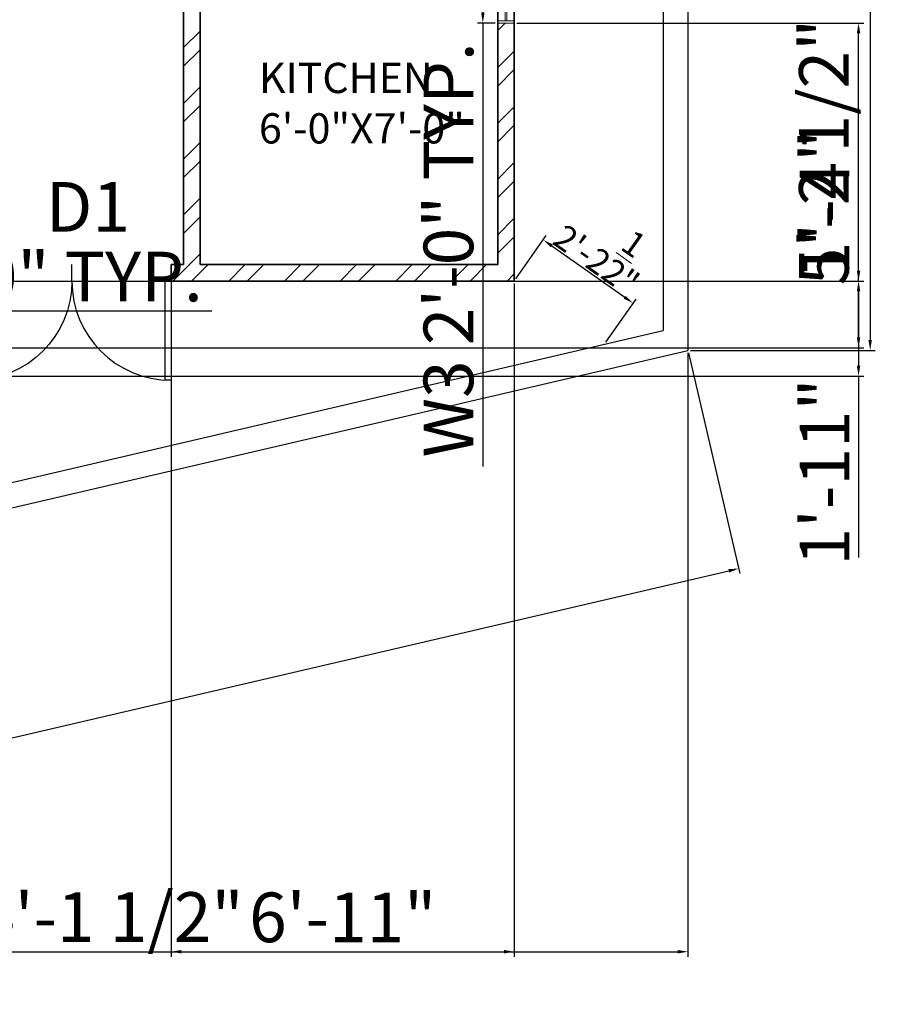
# Model space of a CAD drawing. Units: inches. Extents: x 2242 to 2870, y 1782 to 2635.
# Tile 3 of 7: x 2594 to 2807, y 1782 to 2020. Entities that reach past the tile are written whole.
import ezdxf

# ---------------------------------------------------------------- set-up
doc = ezdxf.new("R2010")
doc.units = ezdxf.units.IN
for name, color, linetype, lineweight in [('A-ANNO-DIMS', 7, 'Continuous', 18), ('A-ANNO-TEXT', 1, 'Continuous', 18), ('A-AREA-IDEN', 1, 'Continuous', 25), ('A-WALL-PATT', 253, 'Continuous', 13), ('C-PROP', 7, 'Continuous', 30), ('doors', 5, 'Continuous', 25), ('walls', 7, 'Continuous', 35), ('windows', 72, 'Continuous', 18)]:
    doc.layers.add(name, color=color, linetype=linetype, lineweight=lineweight)
doc.styles.get("Standard").update_dxf_attribs({"font": 'arial.ttf'})
doc.dimstyles.new('ISO-25', dxfattribs={"dimtxt": 12, "dimasz": 2.5, "dimexe": 1.25, "dimexo": 0.625, "dimtad": 1, "dimlunit": 4, "dimtxsty": 'Standard', "dimcen": 2.5, "dimadec": 0, "dimazin": 0, "dimtfac": 1, "dimtmove": 0, "dimatfit": 3, "dimfxl": 1, "dimarcsym": 0})

# ---------------------------------------------------------------- blocks, each defined once
blk = doc.blocks.new('*U2')
for p, q in [((0, 0), (0, -5)), ((30, 0), (30, -5))]:
    blk.add_line(p, q)
blk.add_lwpolyline([(0, 0), (0, 30), (1.75, 30), (1.75, 0)], close=True)
blk.add_arc((0, 0), 30, 0, 90)
blk = doc.blocks.new('*D17')
at = {"layer": 'A-ANNO-DIMS', "color": 0, "lineweight": -2, "transparency": 16777216}
for p, q in [((2755.31, 1939.73), (2767.74, 1886.37)), ((2322.86, 1784), (2765.02, 1887.02)), ((2308.28, 1835.57), (2320.71, 1782.21))]:
    blk.add_line(p, q, dxfattribs=at)
at = {"layer": 'A-ANNO-DIMS', "color": 0, "transparency": 16777216}
for points in [[(2764.92, 1887.42), (2765.11, 1886.61), (2767.45, 1887.58)], [(2322.77, 1784.4), (2322.96, 1783.59), (2320.43, 1783.43)]]:
    blk.add_solid(points, dxfattribs=at)
at = {"layer": 'Defpoints', "color": 0, "transparency": 16777216}
for p in [(2755.16, 1940.33), (2767.45, 1887.58), (2308.14, 1836.18)]:
    blk.add_point(p, dxfattribs=at)
at = {"layer": 'A-ANNO-DIMS', "color": 0, "transparency": 16777216, "insert": (2542.41, 1842.09), "char_height": 12, "attachment_point": 5, "rotation": 13.1155}
blk.add_mtext('38\'-3"', dxfattribs=at)
blk = doc.blocks.new('*D19')
at = {"layer": 'A-ANNO-DIMS', "color": 0, "lineweight": -2, "transparency": 16777216}
for p, q in [((2713.52, 1957.61), (2720.9, 1968.07)), ((2722.22, 1965.61), (2739.87, 1953.17)), ((2735.26, 1942.28), (2742.64, 1952.75))]:
    blk.add_line(p, q, dxfattribs=at)
at = {"layer": 'A-ANNO-DIMS', "color": 0, "transparency": 16777216}
for points in [[(2722.46, 1965.95), (2721.98, 1965.27), (2720.18, 1967.05)], [(2740.11, 1953.51), (2739.63, 1952.83), (2741.92, 1951.73)]]:
    blk.add_solid(points, dxfattribs=at)
at = {"layer": 'Defpoints', "color": 0, "transparency": 16777216}
for p in [(2713.16, 1957.1), (2741.92, 1951.73), (2734.9, 1941.77)]:
    blk.add_point(p, dxfattribs=at)
at = {"layer": 'A-ANNO-DIMS', "color": 0, "transparency": 16777216, "insert": (2735.46, 1965.64), "char_height": 6, "attachment_point": 5, "rotation": 324.8144}
blk.add_mtext('2\'-2{\\H1x;\\S1/2;}"', dxfattribs=at)
blk = doc.blocks.new('*D29')
at = {"layer": 'A-ANNO-DIMS', "color": 0, "lineweight": -2, "transparency": 16777216}
for p, q in [((2755.79, 2540.33), (2800.47, 2540.33)), ((2799.22, 2537.83), (2799.22, 1942.83)), ((2755.79, 1940.33), (2800.47, 1940.33))]:
    blk.add_line(p, q, dxfattribs=at)
at = {"layer": 'A-ANNO-DIMS', "color": 0, "transparency": 16777216}
for points in [[(2798.81, 2537.83), (2799.64, 2537.83), (2799.22, 2540.33)], [(2798.81, 1942.83), (2799.64, 1942.83), (2799.22, 1940.33)]]:
    blk.add_solid(points, dxfattribs=at)
at = {"layer": 'Defpoints', "color": 0, "transparency": 16777216}
for p in [(2755.16, 2540.33), (2755.16, 1940.33), (2799.22, 1940.33)]:
    blk.add_point(p, dxfattribs=at)
at = {"layer": 'A-ANNO-DIMS', "color": 0, "transparency": 16777216, "insert": (2792.47, 2240.33), "char_height": 12, "attachment_point": 5, "rotation": 90}
blk.add_mtext("50'", dxfattribs=at)
blk = doc.blocks.new('WIN-W3-24IN')
for p, q in [((0, 0), (0, 24.12)), ((0, 24.12), (4, 24.12)), ((4, 24.12), (4, 0)), ((0, 23.62), (4, 23.62)), ((1.8, 23.62), (1.8, 0.5)), ((2.2, 23.62), (2.2, 0.5)), ((4, 0.5), (0, 0.5)), ((4, 0), (0, 0))]:
    blk.add_line(p, q)
blk = doc.blocks.new('*D35')
at = {"layer": 'A-ANNO-DIMS', "color": 0, "lineweight": -2, "transparency": 16777216}
for p, q in [((2484.67, 1956.47), (2484.67, 1948.63)), ((2532.79, 1956.47), (2532.79, 1948.63)), ((2487.17, 1949.88), (2530.29, 1949.88)), ((2532.79, 1949.88), (2639.98, 1949.88))]:
    blk.add_line(p, q, dxfattribs=at)
at = {"layer": 'A-ANNO-DIMS', "color": 0, "transparency": 16777216}
for points in [[(2487.17, 1950.3), (2487.17, 1949.46), (2484.67, 1949.88)], [(2530.29, 1950.3), (2530.29, 1949.46), (2532.79, 1949.88)]]:
    blk.add_solid(points, dxfattribs=at)
at = {"layer": 'Defpoints', "color": 0, "transparency": 16777216}
for p in [(2484.67, 1957.1), (2532.79, 1957.1), (2532.79, 1949.88)]:
    blk.add_point(p, dxfattribs=at)
at = {"layer": 'A-ANNO-DIMS', "color": 0, "transparency": 16777216, "insert": (2587.64, 1956.63), "char_height": 12, "attachment_point": 5}
blk.add_mtext('W1 4\'-0" TYP.', dxfattribs=at)
blk = doc.blocks.new('*D37')
at = {"layer": 'A-ANNO-DIMS', "color": 0, "lineweight": -2, "transparency": 16777216}
for p, q in [((2708.54, 2043.59), (2704.3, 2043.59)), ((2705.55, 2041.09), (2705.55, 2021.98)), ((2708.54, 2019.48), (2704.3, 2019.48)), ((2705.55, 2019.48), (2705.55, 1912.29))]:
    blk.add_line(p, q, dxfattribs=at)
at = {"layer": 'A-ANNO-DIMS', "color": 0, "transparency": 16777216}
for points in [[(2705.13, 2041.09), (2705.96, 2041.09), (2705.55, 2043.59)], [(2705.13, 2021.98), (2705.96, 2021.98), (2705.55, 2019.48)]]:
    blk.add_solid(points, dxfattribs=at)
at = {"layer": 'Defpoints', "color": 0, "transparency": 16777216}
for p in [(2709.16, 2043.59), (2705.55, 2019.48), (2709.16, 2019.48)]:
    blk.add_point(p, dxfattribs=at)
at = {"layer": 'A-ANNO-DIMS', "color": 0, "transparency": 16777216, "insert": (2698.79, 1964.63), "char_height": 12, "attachment_point": 5, "rotation": 90}
blk.add_mtext('W3 2\'-0" TYP.', dxfattribs=at)
blk = doc.blocks.new('*D42')
at = {"layer": 'A-ANNO-DIMS', "color": 0, "lineweight": -2, "transparency": 16777216}
for p, q in [((2522.93, 2020.21), (2522.93, 2026.94)), ((2537.42, 2020.21), (2537.42, 2026.94)), ((2525.43, 2025.69), (2534.92, 2025.69)), ((2537.42, 2025.69), (2641.15, 2025.69))]:
    blk.add_line(p, q, dxfattribs=at)
at = {"layer": 'A-ANNO-DIMS', "color": 0, "transparency": 16777216}
for points in [[(2525.43, 2026.11), (2525.43, 2025.28), (2522.93, 2025.69)], [(2534.92, 2026.11), (2534.92, 2025.28), (2537.42, 2025.69)]]:
    blk.add_solid(points, dxfattribs=at)
at = {"layer": 'Defpoints', "color": 0, "transparency": 16777216}
for p in [(2537.42, 2025.69), (2522.93, 2019.58), (2537.42, 2019.58)]:
    blk.add_point(p, dxfattribs=at)
at = {"layer": 'A-ANNO-DIMS', "color": 0, "transparency": 16777216, "insert": (2590.54, 2032.52), "char_height": 12, "attachment_point": 5}
blk.add_mtext('1\'-2 1/2" TYP.', dxfattribs=at)
blk = doc.blocks.new('*D56')
at = {"layer": 'A-ANNO-DIMS', "color": 0, "lineweight": -2, "transparency": 16777216}
for p, q in [((2755.16, 1939.71), (2755.16, 1793.68)), ((2308.14, 1835.56), (2308.14, 1793.68)), ((2310.64, 1794.93), (2752.66, 1794.93))]:
    blk.add_line(p, q, dxfattribs=at)
at = {"layer": 'A-ANNO-DIMS', "color": 0, "transparency": 16777216}
for points in [[(2310.64, 1795.35), (2310.64, 1794.51), (2308.14, 1794.93)], [(2752.66, 1795.35), (2752.66, 1794.51), (2755.16, 1794.93)]]:
    blk.add_solid(points, dxfattribs=at)
at = {"layer": 'Defpoints', "color": 0, "transparency": 16777216}
for p in [(2755.16, 1940.33), (2308.14, 1836.18), (2755.16, 1794.93)]:
    blk.add_point(p, dxfattribs=at)
at = {"layer": 'A-ANNO-DIMS', "color": 0, "transparency": 16777216, "insert": (2531.65, 1801.69), "char_height": 12, "attachment_point": 5}
blk.add_mtext('37\'-3"', dxfattribs=at)
blk = doc.blocks.new('*D57')
at = {"layer": 'A-ANNO-DIMS', "color": 0, "lineweight": -2, "transparency": 16777216}
for p, q in [((2713.16, 1956.47), (2713.16, 1793.68)), ((2388.74, 1896.47), (2388.74, 1793.68)), ((2391.24, 1794.93), (2710.66, 1794.93))]:
    blk.add_line(p, q, dxfattribs=at)
at = {"layer": 'A-ANNO-DIMS', "color": 0, "transparency": 16777216}
for points in [[(2391.24, 1795.35), (2391.24, 1794.51), (2388.74, 1794.93)], [(2710.66, 1795.35), (2710.66, 1794.51), (2713.16, 1794.93)]]:
    blk.add_solid(points, dxfattribs=at)
at = {"layer": 'Defpoints', "color": 0, "transparency": 16777216}
for p in [(2713.16, 1957.1), (2388.74, 1897.1), (2713.16, 1794.93)]:
    blk.add_point(p, dxfattribs=at)
at = {"layer": 'A-ANNO-DIMS', "color": 0, "transparency": 16777216, "insert": (2550.95, 1801.76), "char_height": 12, "attachment_point": 5}
blk.add_mtext('27\'-0 1/2"', dxfattribs=at)
blk = doc.blocks.new('*D68')
at = {"layer": 'A-ANNO-DIMS', "color": 0, "lineweight": -2, "transparency": 16777216}
for p, q in [((2713.79, 2019.48), (2797.66, 2019.48)), ((2796.41, 1959.6), (2796.41, 2016.98)), ((2713.79, 1957.1), (2797.66, 1957.1))]:
    blk.add_line(p, q, dxfattribs=at)
at = {"layer": 'A-ANNO-DIMS', "color": 0, "transparency": 16777216}
for points in [[(2796, 2016.98), (2796.83, 2016.98), (2796.41, 2019.48)], [(2796, 1959.6), (2796.83, 1959.6), (2796.41, 1957.1)]]:
    blk.add_solid(points, dxfattribs=at)
at = {"layer": 'Defpoints', "color": 0, "transparency": 16777216}
for p in [(2713.16, 2019.48), (2796.41, 2019.48), (2713.16, 1957.1)]:
    blk.add_point(p, dxfattribs=at)
at = {"layer": 'A-ANNO-DIMS', "color": 0, "transparency": 16777216, "insert": (2789.58, 1988.29), "char_height": 12, "attachment_point": 5, "rotation": 90}
blk.add_mtext('5\'-2 1/2"', dxfattribs=at)
blk = doc.blocks.new('*D72')
at = {"layer": 'A-ANNO-DIMS', "color": 0, "lineweight": -2, "transparency": 16777216}
for p, q in [((2532.79, 1956.47), (2532.79, 1793.68)), ((2582.16, 1956.47), (2582.16, 1793.68)), ((2535.29, 1794.93), (2579.66, 1794.93)), ((2582.16, 1794.93), (2646.26, 1794.93))]:
    blk.add_line(p, q, dxfattribs=at)
at = {"layer": 'A-ANNO-DIMS', "color": 0, "transparency": 16777216}
for points in [[(2535.29, 1795.35), (2535.29, 1794.51), (2532.79, 1794.93)], [(2579.66, 1795.35), (2579.66, 1794.51), (2582.16, 1794.93)]]:
    blk.add_solid(points, dxfattribs=at)
at = {"layer": 'Defpoints', "color": 0, "transparency": 16777216}
for p in [(2532.79, 1957.1), (2582.16, 1957.1), (2582.16, 1794.93)]:
    blk.add_point(p, dxfattribs=at)
at = {"layer": 'A-ANNO-DIMS', "color": 0, "transparency": 16777216, "insert": (2615.46, 1801.76), "char_height": 12, "attachment_point": 5}
blk.add_mtext('4\'-1 1/2"', dxfattribs=at)
blk = doc.blocks.new('*D73')
at = {"layer": 'A-ANNO-DIMS', "color": 0, "lineweight": -2, "transparency": 16777216}
for p, q in [((2630.16, 1956.47), (2630.16, 1793.68)), ((2713.16, 1956.47), (2713.16, 1793.68)), ((2632.66, 1794.93), (2710.66, 1794.93))]:
    blk.add_line(p, q, dxfattribs=at)
at = {"layer": 'A-ANNO-DIMS', "color": 0, "transparency": 16777216}
for points in [[(2632.66, 1795.35), (2632.66, 1794.51), (2630.16, 1794.93)], [(2710.66, 1795.35), (2710.66, 1794.51), (2713.16, 1794.93)]]:
    blk.add_solid(points, dxfattribs=at)
at = {"layer": 'Defpoints', "color": 0, "transparency": 16777216}
for p in [(2630.16, 1957.1), (2713.16, 1957.1), (2713.16, 1794.93)]:
    blk.add_point(p, dxfattribs=at)
at = {"layer": 'A-ANNO-DIMS', "color": 0, "transparency": 16777216, "insert": (2671.66, 1801.68), "char_height": 12, "attachment_point": 5}
blk.add_mtext('6\'-11"', dxfattribs=at)
blk = doc.blocks.new('*D76')
at = {"layer": 'A-ANNO-DIMS', "color": 0, "lineweight": -2, "transparency": 16777216}
for p, q in [((2796.41, 1957.1), (2796.41, 1991.62)), ((2393.37, 1957.1), (2797.66, 1957.1)), ((2796.41, 1943.45), (2796.41, 1954.6)), ((2393.37, 1940.95), (2797.66, 1940.95))]:
    blk.add_line(p, q, dxfattribs=at)
at = {"layer": 'A-ANNO-DIMS', "color": 0, "transparency": 16777216}
for points in [[(2796, 1954.6), (2796.83, 1954.6), (2796.41, 1957.1)], [(2796, 1943.45), (2796.83, 1943.45), (2796.41, 1940.95)]]:
    blk.add_solid(points, dxfattribs=at)
at = {"layer": 'Defpoints', "color": 0, "transparency": 16777216}
for p in [(2392.74, 1957.1), (2796.41, 1957.1), (2392.74, 1940.95)]:
    blk.add_point(p, dxfattribs=at)
at = {"layer": 'A-ANNO-DIMS', "color": 0, "transparency": 16777216, "insert": (2789.76, 1975.61), "char_height": 12, "attachment_point": 5, "rotation": 90}
blk.add_mtext('1\'-4"', dxfattribs=at)
blk = doc.blocks.new('*D85')
at = {"layer": 'A-ANNO-DIMS', "color": 0, "lineweight": -2, "transparency": 16777216}
for p, q in [((2465.37, 1957.1), (2797.66, 1957.1)), ((2796.41, 1954.6), (2796.41, 1936.6)), ((2465.37, 1934.1), (2797.66, 1934.1)), ((2796.41, 1934.1), (2796.41, 1890.25))]:
    blk.add_line(p, q, dxfattribs=at)
at = {"layer": 'A-ANNO-DIMS', "color": 0, "transparency": 16777216}
for points in [[(2796, 1954.6), (2796.83, 1954.6), (2796.41, 1957.1)], [(2796, 1936.6), (2796.83, 1936.6), (2796.41, 1934.1)]]:
    blk.add_solid(points, dxfattribs=at)
at = {"layer": 'Defpoints', "color": 0, "transparency": 16777216}
for p in [(2464.74, 1957.1), (2464.74, 1934.1), (2796.41, 1934.1)]:
    blk.add_point(p, dxfattribs=at)
at = {"layer": 'A-ANNO-DIMS', "color": 0, "transparency": 16777216, "insert": (2789.76, 1910.93), "char_height": 12, "attachment_point": 5, "rotation": 90}
blk.add_mtext('1\'-11"', dxfattribs=at)

msp = doc.modelspace()

# ---------------------------------------------------------------- hatches: boundary and pattern name
at = {"layer": 'A-WALL-PATT'}
h = msp.add_hatch(dxfattribs=at)
h.set_pattern_fill('ANSI32', color=256)
h.paths.add_polyline_path([(2713.164, 2019.476), (2709.164, 2019.476), (2709.164, 1961.097), (2637.164, 1961.097), (2637.164, 2045.097), (2642.164, 2045.097), (2642.164, 2049.097), (2633.164, 2049.097), (2633.164, 1961.097), (2630.164, 1961.097), (2630.164, 1957.097), (2713.164, 1957.097)])

# ---------------------------------------------------------------- linework, layer by layer
at = {"layer": 'C-PROP'}
for p, q in [((2755.164, 2540.335), (2755.164, 1940.335)), ((2749.164, 2534.335), (2749.164, 1945.097)), ((2314.71, 1843.873), (2749.164, 1945.097)), ((2308.137, 1836.181), (2755.164, 1940.335))]:
    msp.add_line(p, q, dxfattribs=at)
at = {"layer": 'walls'}
for p, q in [((2709.164, 2254.097), (2709.164, 1961.097)), ((2713.164, 2254.097), (2713.164, 1957.097)), ((2633.164, 2049.097), (2633.164, 1961.097)), ((2637.164, 2045.097), (2637.164, 1961.097)), ((2633.164, 1961.097), (2630.164, 1961.097)), ((2630.164, 1961.097), (2630.164, 1957.097)), ((2633.164, 1961.097), (2630.164, 1961.097)), ((2709.164, 1961.097), (2637.164, 1961.097)), ((2713.164, 1957.097), (2630.164, 1957.097)), ((2642.164, 1957.097), (2630.164, 1957.097))]:
    msp.add_line(p, q, dxfattribs=at)

# ---------------------------------------------------------------- block references
at = {"layer": 'doors', "yscale": 0.8, "zscale": 0.8, "rotation": 180}
for p, xscale in [((2582.164, 1957.097), -0.8), ((2630.164, 1957.097), 0.8)]:
    msp.add_blockref('*U2', p, dxfattribs=dict(at, xscale=xscale))
at = {"layer": 'windows', "rotation": 180}
msp.add_blockref('WIN-W3-24IN', (2713.163, 2043.592), dxfattribs=at)

# ---------------------------------------------------------------- texts
at = {"layer": 'A-ANNO-TEXT', "insert": (2599.863, 1981.029), "char_height": 12, "attachment_point": 1}
msp.add_mtext_dynamic_manual_height_columns('D1', width=2.16795, gutter_width=12.5, heights=[0], dxfattribs=at)
at = {"layer": 'A-AREA-IDEN', "insert": (2651.394, 2009.857), "char_height": 7.31253, "attachment_point": 1}
msp.add_mtext_dynamic_manual_height_columns('KITCHEN\\P6\'-0"X7\'-0"', width=0.7828, gutter_width=36.563, heights=[0], dxfattribs=at)

# ---------------------------------------------------------------- dimensions: what is measured, and where the dimension line sits
at = {"layer": 'A-ANNO-DIMS'}
for base, p1, p2, override, picture, middle in [((2799.223, 1940.335), (2755.164, 2540.335), (2755.164, 1940.335), {"dimclrd": 0, "dimclre": 0, "dimclrt": 0}, '*D29', (2792.471, 2240.335)), ((2796.414, 2019.476), (2713.164, 1957.097), (2713.164, 2019.476), {"dimdec": 1, "dimlfac": 1, "dimrnd": 0, "dimzin": 1, "dimdsep": 46, "dimlunit": 4, "dimfrac": 2}, '*D68', (2789.584, 1988.287)), ((2796.414, 1957.097), (2392.745, 1940.946), (2392.745, 1957.097), {"dimdec": 1, "dimlfac": 1, "dimrnd": 0, "dimzin": 1, "dimdsep": 46, "dimlunit": 4, "dimfrac": 2}, '*D76', (2789.764, 1975.607)), ((2796.414, 1934.097), (2464.745, 1957.097), (2464.745, 1934.097), {"dimdec": 1, "dimlfac": 1, "dimrnd": 0, "dimzin": 1, "dimdsep": 46, "dimlunit": 4, "dimfrac": 2}, '*D85', (2789.764, 1910.926))]:
    dim = msp.add_linear_dim(base=base, p1=p1, p2=p2, angle=90, dimstyle='ISO-25', override=override, dxfattribs=at)
    dim.commit()
    dim.dimension.update_dxf_attribs({"geometry": picture, "text_midpoint": middle})
for base, p1, p2, text, picture, middle in [((2537.424, 2025.694), (2522.931, 2019.58), (2537.424, 2019.58), '<> TYP.', '*D42', (2590.538, 2032.524)), ((2532.79, 1949.88), (2484.674, 1957.097), (2532.79, 1957.097), 'W1 <> TYP.', '*D35', (2587.635, 1956.632))]:
    dim = msp.add_linear_dim(base=base, p1=p1, p2=p2, text=text, dimstyle='ISO-25', override={"dimdec": 1, "dimlfac": 1, "dimrnd": 0, "dimzin": 1, "dimdsep": 46, "dimlunit": 4, "dimfrac": 2}, dxfattribs=at)
    dim.commit()
    dim.dimension.update_dxf_attribs({"geometry": picture, "text_midpoint": middle})
dim = msp.add_linear_dim(base=(2705.546, 2019.476), p1=(2709.164, 2043.592), p2=(2709.164, 2019.476), angle=270, text='W3 <> TYP.', dimstyle='ISO-25', override={"dimdec": 1, "dimlfac": 1, "dimrnd": 0, "dimzin": 1, "dimdsep": 46, "dimlunit": 4, "dimfrac": 2}, dxfattribs=at)
dim.commit()
dim.dimension.update_dxf_attribs({"geometry": '*D37', "text_midpoint": (2698.79, 1964.631)})
for p1, p2, distance, override, picture, middle in [((2713.164, 1957.097), (2734.898, 1941.774), 12.179, {"dimtxt": 6, "dimclrd": 0, "dimclre": 0, "dimclrt": 0}, '*D19', (2735.456, 1965.641)), ((2308.137, 1836.181), (2755.164, 1940.335), -54.163, {"dimclrd": 0, "dimclre": 0, "dimclrt": 0}, '*D17', (2542.407, 1842.087))]:
    dim = msp.add_aligned_dim(p1=p1, p2=p2, distance=distance, dimstyle='ISO-25', override=override, dxfattribs=at)
    dim.commit()
    dim.dimension.update_dxf_attribs({"geometry": picture, "text_midpoint": middle})
for base, p1, p2, picture, middle in [((2713.164, 1794.931), (2388.745, 1897.097), (2713.164, 1957.097), '*D57', (2550.954, 1801.761)), ((2582.164, 1794.931), (2532.79, 1957.097), (2582.164, 1957.097), '*D72', (2615.46, 1801.761)), ((2713.164, 1794.931), (2630.164, 1957.097), (2713.164, 1957.097), '*D73', (2671.664, 1801.683)), ((2755.164, 1794.931), (2308.137, 1836.181), (2755.164, 1940.335), '*D56', (2531.65, 1801.687))]:
    dim = msp.add_linear_dim(base=base, p1=p1, p2=p2, dimstyle='ISO-25', override={"dimdec": 1, "dimlfac": 1, "dimrnd": 0, "dimzin": 1, "dimdsep": 46, "dimlunit": 4, "dimfrac": 2}, dxfattribs=at)
    dim.commit()
    dim.dimension.update_dxf_attribs({"geometry": picture, "text_midpoint": middle})

doc.saveas('drawing.dxf')
